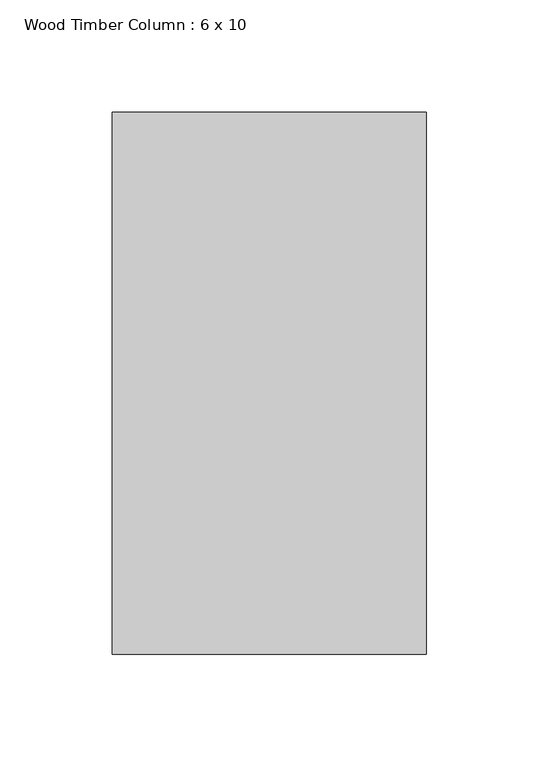
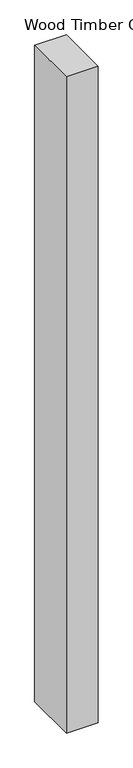
"""IFC4 building model written with IfcOpenShell, lengths in millimetres: column geometry, Wood Timber Column : 6 x 10."""

from ifc_helpers import new_model, si_unit, origin, origin_with_axes, place, context, project, spatial, polyline, outline, extrude, source, transform, mapped, element, save


def wood_timber_column_6_x_10_8585acab(model_context):
    return source(origin(), model_context, "Body", "SweptSolid", [
        extrude(outline(polyline([(69.85, -120.65), (-69.85, -120.65), (-69.85, 120.65), (69.85, 120.65), (69.85, -120.65)])), origin_with_axes(), (0.0, 0.0, 1.0), 3048.0),
    ])


if __name__ == "__main__":
    model = new_model("IFC4")
    model_context = context("Model", 3, world=origin())
    ifc_project = project(units=[si_unit("LENGTHUNIT", "METRE", prefix="MILLI")], contexts=[model_context])
    site = spatial("IfcSite", under=ifc_project)
    building = spatial("IfcBuilding", under=site)
    placement = place(None, origin())
    wood_timber_column_6_x_10_shape = wood_timber_column_6_x_10_8585acab(model_context)
    element("IfcColumn", 1, ObjectType="Wood Timber Column : 6 x 10", at=placement, inside=building, context=model_context, shape_type="MappedRepresentation", body=[
        mapped(wood_timber_column_6_x_10_shape, transform((0.0, 0.0, 0.0), x_axis=(1.0, 0.0, 0.0), y_axis=(0.0, 1.0, 0.0), z_axis=(0.0, 0.0, 1.0))),
    ])
    save(model, "model.ifc")

# Revit data of these elements
# Type "Wood Timber Column : 6 x 10"
#   Assembly Code = "B1010200"
#   Depth = 0' - 9 1/2"
#   Width = 0' - 5 1/2"
#   Material = Softwood, Lumber
# Element 1 (IfcColumn, "Wood Timber Column : 6 x 10")
#   Materials on its faces: "Softwood, Lumber"
# Materials
#   "Softwood, Lumber": class "Wood", colour RGB 223 192 134, transparency 0, Description = "Pinus Echinata", Cost = 0
